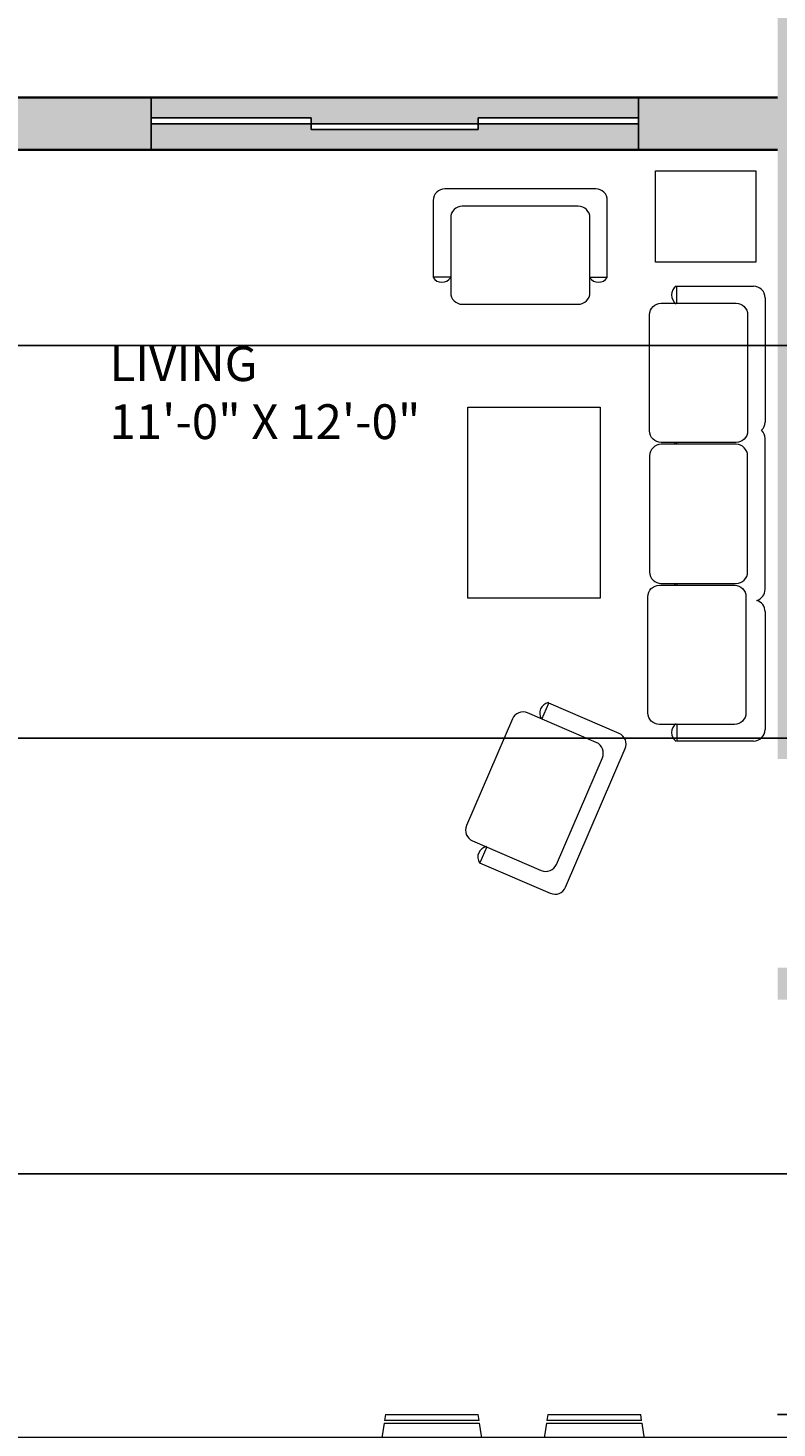
# Model space of a CAD drawing. Units: inches. Extents: x 1693 to 2974, y 2201 to 2965.
# Tile 21 of 24: x 2628 to 2757, y 2588 to 2829. Entities that reach past the tile are written whole.
import ezdxf

# ---------------------------------------------------------------- set-up
doc = ezdxf.new("R2010")
doc.units = ezdxf.units.IN
doc.header["$LTSCALE"] = 2
doc.header["$MEASUREMENT"] = 0
for name, color, linetype, lineweight in [('A-ANNO-DIMS', 2, 'Continuous', 18), ('A-AREA-IDEN', 7, 'Continuous', 18), ('A-DOOR', 3, 'Continuous', 25), ('A-FURN', 8, 'Continuous', 18), ('A-WALL', 7, 'Continuous', 35)]:
    doc.layers.add(name, color=color, linetype=linetype, lineweight=lineweight)
doc.layers.add('A-GLAZ-PATT', color=141, linetype='Continuous', lineweight=13, true_color=0xadddf7)
doc.layers.add('A-WALL-PATT', color=251, linetype='Continuous', lineweight=13, true_color=0x636466)
doc.styles.get("Standard").update_dxf_attribs({"font": 'arial.ttf'})
doc.dimstyles.get("Standard").update_dxf_attribs({"dimtxt": 0.18, "dimasz": 0.18, "dimexe": 0.18, "dimexo": 0.0625, "dimgap": 0.09, "dimtad": 0, "dimtih": 1, "dimtoh": 1, "dimdec": 1, "dimzin": 0, "dimdsep": 46, "dimlunit": 3, "dimtxsty": 'Standard', "dimcen": 0.09, "dimadec": 0, "dimazin": 0, "dimtfac": 1, "dimtdec": 1, "dimtofl": 0, "dimtmove": 0, "dimatfit": 3, "dimfxl": 1, "dimtolj": 1, "dimtzin": 0, "dimarcsym": 0})

# ---------------------------------------------------------------- blocks, each defined once
blk = doc.blocks.new('DINING-SET-72x36-6-SEAT')
for p, q in [((23.27, 53.5), (22.02, 45.5)), ((23.27, 53.5), (39.74, 53.5)), ((23.5, 55), (23.34, 54)), ((39.66, 54), (23.35, 54)), ((23.5, 55), (39.5, 55)), ((39.66, 54), (39.5, 55)), ((40.98, 45.5), (39.73, 53.5)), ((51.27, 53.5), (50.02, 45.5)), ((51.27, 53.5), (67.74, 53.5)), ((51.5, 55), (51.34, 54)), ((67.66, 54), (51.35, 54)), ((51.5, 55), (67.5, 55)), ((67.66, 54), (67.5, 55)), ((68.98, 45.5), (67.73, 53.5)), ((81.5, 45.5), (9.5, 45.5)), ((9.5, 45.5), (9.5, 9.5)), ((81.5, 9.5), (81.5, 45.5)), ((1.5, 35.73), (9.5, 36.98)), ((89.5, 35.73), (81.5, 36.98)), ((0, 35.5), (1, 35.66)), ((0, 35.5), (0, 19.5)), ((1, 19.34), (1, 35.65)), ((1.5, 35.73), (1.5, 19.26)), ((89.5, 35.73), (89.5, 19.26)), ((91, 35.5), (90, 35.66)), ((90, 19.34), (90, 35.65)), ((91, 35.5), (91, 19.5)), ((1, 19.34), (0, 19.5)), ((90, 19.34), (91, 19.5)), ((9.5, 18.02), (1.5, 19.27)), ((81.5, 18.02), (89.5, 19.27)), ((9.5, 9.5), (81.5, 9.5)), ((23.27, 1.5), (22.02, 9.5)), ((40.98, 9.5), (39.73, 1.5)), ((51.27, 1.5), (50.02, 9.5)), ((68.98, 9.5), (67.73, 1.5)), ((23.27, 1.5), (39.74, 1.5)), ((23.5, 0), (23.34, 1)), ((39.66, 1), (23.35, 1)), ((23.5, 0), (39.5, 0)), ((39.66, 1), (39.5, 0)), ((51.27, 1.5), (67.74, 1.5)), ((51.5, 0), (51.34, 1)), ((67.66, 1), (51.35, 1)), ((51.5, 0), (67.5, 0)), ((67.66, 1), (67.5, 0))]:
    blk.add_line(p, q)
blk = doc.blocks.new('*D62')
at = {"layer": 'A-ANNO-DIMS', "color": 0, "lineweight": -2, "ltscale": 2, "transparency": 16777216}
for p, q in [((2756.69, 2590.25), (2770.46, 2590.25)), ((2770.28, 2590.07), (2770.28, 2562.93)), ((2770.28, 2535.43), (2770.28, 2562.56)), ((2756.69, 2535.25), (2770.46, 2535.25))]:
    blk.add_line(p, q, dxfattribs=at)
at = {"layer": 'A-ANNO-DIMS', "color": 0, "ltscale": 2, "transparency": 16777216}
for points in [[(2770.25, 2590.07), (2770.31, 2590.07), (2770.28, 2590.25)], [(2770.25, 2535.43), (2770.31, 2535.43), (2770.28, 2535.25)]]:
    blk.add_solid(points, dxfattribs=at)
at = {"layer": 'Defpoints', "color": 0, "ltscale": 2, "transparency": 16777216}
for p in [(2756.63, 2590.25), (2770.28, 2590.25), (2756.63, 2535.25)]:
    blk.add_point(p, dxfattribs=at)
at = {"layer": 'A-ANNO-DIMS', "color": 0, "ltscale": 2, "transparency": 16777216, "insert": (2770.28, 2562.75), "char_height": 0.18, "attachment_point": 5}
blk.add_mtext('\\A1;55 TYP.', dxfattribs=at)
blk = doc.blocks.new('*D81')
at = {"layer": 'A-ANNO-DIMS', "color": 0, "lineweight": -2, "ltscale": 2, "transparency": 16777216}
for p, q in [((1752.34, 2553.91), (1752.34, 2964.96)), ((1752.52, 2964.78), (2332.94, 2964.78)), ((2914.06, 2964.78), (2333.64, 2964.78)), ((2914.24, 2754.97), (2914.24, 2964.96))]:
    blk.add_line(p, q, dxfattribs=at)
at = {"layer": 'A-ANNO-DIMS', "color": 0, "ltscale": 2, "transparency": 16777216}
for points in [[(1752.52, 2964.81), (1752.52, 2964.75), (1752.34, 2964.78)], [(2914.06, 2964.81), (2914.06, 2964.75), (2914.24, 2964.78)]]:
    blk.add_solid(points, dxfattribs=at)
at = {"layer": 'Defpoints', "color": 0, "ltscale": 2, "transparency": 16777216}
for p in [(2914.24, 2964.78), (2914.24, 2754.9), (1752.34, 2553.84)]:
    blk.add_point(p, dxfattribs=at)
at = {"layer": 'A-ANNO-DIMS', "color": 0, "ltscale": 2, "transparency": 16777216, "insert": (2333.29, 2964.78), "char_height": 0.18, "attachment_point": 5}
blk.add_mtext('\\A1;1162', dxfattribs=at)
blk = doc.blocks.new('*D90')
at = {"layer": 'A-ANNO-DIMS', "color": 0, "lineweight": -2, "ltscale": 2, "transparency": 16777216}
for p, q in [((2145.8, 2774.54), (2973.12, 2774.54)), ((2972.94, 2774.36), (2972.94, 2740.87)), ((2972.94, 2707.02), (2972.94, 2740.51)), ((2294.3, 2706.84), (2973.12, 2706.84))]:
    blk.add_line(p, q, dxfattribs=at)
at = {"layer": 'A-ANNO-DIMS', "color": 0, "ltscale": 2, "transparency": 16777216}
for points in [[(2972.91, 2774.36), (2972.97, 2774.36), (2972.94, 2774.54)], [(2972.91, 2707.02), (2972.97, 2707.02), (2972.94, 2706.84)]]:
    blk.add_solid(points, dxfattribs=at)
at = {"layer": 'Defpoints', "color": 0, "ltscale": 2, "transparency": 16777216}
for p in [(2145.74, 2774.54), (2294.24, 2706.84), (2972.94, 2706.84)]:
    blk.add_point(p, dxfattribs=at)
at = {"layer": 'A-ANNO-DIMS', "color": 0, "ltscale": 2, "transparency": 16777216, "insert": (2972.94, 2740.69), "char_height": 0.18, "attachment_point": 5}
blk.add_mtext('\\A1;67.7', dxfattribs=at)
blk = doc.blocks.new('*D97')
at = {"layer": 'A-ANNO-DIMS', "color": 0, "lineweight": -2, "ltscale": 2, "transparency": 16777216}
for p, q in [((2294.3, 2631.75), (2973.12, 2631.75)), ((2972.94, 2631.57), (2972.94, 2609.19)), ((2972.94, 2586.44), (2972.94, 2608.83)), ((2294.3, 2586.26), (2973.12, 2586.26))]:
    blk.add_line(p, q, dxfattribs=at)
at = {"layer": 'A-ANNO-DIMS', "color": 0, "ltscale": 2, "transparency": 16777216}
for points in [[(2972.91, 2631.57), (2972.97, 2631.57), (2972.94, 2631.75)], [(2972.91, 2586.44), (2972.97, 2586.44), (2972.94, 2586.26)]]:
    blk.add_solid(points, dxfattribs=at)
at = {"layer": 'Defpoints', "color": 0, "ltscale": 2, "transparency": 16777216}
for p in [(2294.24, 2631.75), (2972.94, 2631.75), (2294.24, 2586.26)]:
    blk.add_point(p, dxfattribs=at)
at = {"layer": 'A-ANNO-DIMS', "color": 0, "ltscale": 2, "transparency": 16777216, "insert": (2972.94, 2609.01), "char_height": 0.18, "attachment_point": 5}
blk.add_mtext('\\A1;45.49', dxfattribs=at)

msp = doc.modelspace()

# ---------------------------------------------------------------- hatches: boundary and pattern name
at = {"layer": 'A-GLAZ-PATT', "ltscale": 2}
h = msp.add_hatch(color=256, dxfattribs=at)
h.dxf.hatch_style = 1
h.paths.add_polyline_path([(2656.9702, 2338.2547), (2632.9702, 2338.2547), (2632.9702, 2339.2547), (2608.9702, 2339.2547), (2608.9702, 2334.7547), (2656.9702, 2334.7547)])
h.paths.add_polyline_path([(2656.9702, 2343.7547), (2608.9702, 2343.7547), (2608.9702, 2340.2547), (2632.9702, 2340.2547), (2632.9702, 2339.2547), (2656.9702, 2339.2547)])
h.paths.add_polyline_path([(2775.7544, 2338.2547), (2751.7544, 2338.2547), (2751.7544, 2334.7547), (2775.7544, 2334.7547)])
h.paths.add_polyline_path([(2775.7544, 2343.7547), (2751.7544, 2343.7547), (2751.7544, 2340.2547), (2775.7544, 2340.2547)])
h.paths.add_polyline_path([(2897.7363, 2568.7999), (2893.2363, 2568.7999), (2893.2363, 2520.7999), (2896.7363, 2520.7999), (2896.7363, 2544.7999), (2897.7363, 2544.7999)])
h.paths.add_polyline_path([(2902.2363, 2568.7999), (2898.7363, 2568.7999), (2898.7363, 2544.7999), (2897.7363, 2544.7999), (2897.7363, 2520.7999), (2902.2363, 2520.7999)])
h.paths.add_polyline_path([(2902.2363, 2637.7547), (2898.7363, 2637.7547), (2898.7363, 2613.7547), (2902.2363, 2613.7547)])
h.paths.add_polyline_path([(2896.7363, 2637.7547), (2893.2363, 2637.7547), (2893.2363, 2613.7547), (2896.7363, 2613.7547)])
h.paths.add_polyline_path([(2902.2363, 2748.903), (2899.0477, 2748.903), (2899.0477, 2724.903), (2898.0477, 2724.903), (2898.0477, 2700.903), (2902.2363, 2700.903)])
h.paths.add_polyline_path([(2898.0477, 2748.903), (2893.2363, 2748.903), (2893.2363, 2700.903), (2897.0477, 2700.903), (2897.0477, 2724.903), (2898.0477, 2724.903)])
h.paths.add_polyline_path([(2851.2363, 2846.2547), (2803.2363, 2846.2547), (2803.2363, 2842.7547), (2827.2363, 2842.7547), (2827.2363, 2841.7547), (2851.2363, 2841.7547)])
h.paths.add_polyline_path([(2851.2363, 2840.7547), (2827.2363, 2840.7547), (2827.2363, 2841.7547), (2803.2363, 2841.7547), (2803.2363, 2837.2547), (2851.2363, 2837.2547)])
h.paths.add_polyline_path([(2578.2363, 2846.2547), (2530.2363, 2846.2547), (2530.2363, 2842.7547), (2554.2363, 2842.7547), (2554.2363, 2841.7547), (2578.2363, 2841.7547)])
h.paths.add_polyline_path([(2578.2363, 2840.7547), (2554.2363, 2840.7547), (2554.2363, 2841.7547), (2530.2363, 2841.7547), (2530.2363, 2837.2547), (2578.2363, 2837.2547)])
h.paths.add_polyline_path([(2732.7363, 2812.7547), (2705.1363, 2812.7547), (2705.1363, 2811.7547), (2676.3363, 2811.7547), (2676.3363, 2812.7547), (2648.7363, 2812.7547), (2648.7363, 2808.2547), (2732.7363, 2808.2547)])
h.paths.add_polyline_path([(2732.7363, 2817.2547), (2648.7363, 2817.2547), (2648.7363, 2813.7547), (2676.3363, 2813.7547), (2676.3363, 2812.7547), (2705.1363, 2812.7547), (2705.1363, 2813.7547), (2732.7363, 2813.7547)])
h.paths.add_polyline_path([(2488.2363, 2695.8203), (2484.7878, 2695.8203), (2484.7878, 2671.8203), (2488.2363, 2671.8203)])
h.paths.add_polyline_path([(2482.7878, 2695.8203), (2479.2363, 2695.8203), (2479.2363, 2671.8203), (2482.7878, 2671.8203)])
h.paths.add_polyline_path([(2488.2363, 2572.4371), (2484.7363, 2572.4371), (2484.7363, 2541.4371), (2483.7363, 2541.4371), (2483.7363, 2512.4371), (2488.2363, 2512.4371)])
h.paths.add_polyline_path([(2482.7363, 2541.4371), (2483.7363, 2541.4371), (2483.7363, 2572.4371), (2479.2363, 2572.4371), (2479.2363, 2512.4371), (2482.7363, 2512.4371)])
h.paths.add_polyline_path([(2248.9863, 2706.8449), (2190.9863, 2706.8449), (2190.9863, 2703.3449), (2219.9863, 2703.3449), (2219.9863, 2702.3449), (2248.9863, 2702.3449)])
h.paths.add_polyline_path([(2248.9863, 2701.3449), (2219.9863, 2701.3449), (2219.9863, 2702.3449), (2190.9863, 2702.3449), (2190.9863, 2697.8449), (2248.9863, 2697.8449)])
h.paths.add_polyline_path([(2151.9207, 2293.3449), (2127.9207, 2293.3449), (2127.9207, 2289.8449), (2151.9207, 2289.8449)])
h.paths.add_polyline_path([(2151.9207, 2298.8449), (2127.9207, 2298.8449), (2127.9207, 2295.3449), (2151.9207, 2295.3449)])
h.paths.add_polyline_path([(2084.023, 2293.3449), (2066.023, 2293.3449), (2066.023, 2294.3449), (2048.023, 2294.3449), (2048.023, 2289.8449), (2084.023, 2289.8449)])
h.paths.add_polyline_path([(2084.023, 2298.8449), (2048.023, 2298.8449), (2048.023, 2295.3449), (2066.023, 2295.3449), (2066.023, 2294.3449), (2084.023, 2294.3449)])
h.paths.add_polyline_path([(1966.0781, 2293.3449), (1948.0781, 2293.3449), (1948.0781, 2294.3449), (1930.0781, 2294.3449), (1930.0781, 2289.8449), (1966.0781, 2289.8449)])
h.paths.add_polyline_path([(1966.0781, 2298.8449), (1930.0781, 2298.8449), (1930.0781, 2295.3449), (1948.0781, 2295.3449), (1948.0781, 2294.3449), (1966.0781, 2294.3449)])
h.paths.add_polyline_path([(1787.2363, 2403.1922), (1782.7363, 2403.1922), (1782.7363, 2355.1922), (1786.2363, 2355.1922), (1786.2363, 2379.1922), (1787.2363, 2379.1922)])
h.paths.add_polyline_path([(1791.7363, 2403.1922), (1788.2363, 2403.1922), (1788.2363, 2379.1922), (1787.2363, 2379.1922), (1787.2363, 2355.1922), (1791.7363, 2355.1922)])
h.paths.add_polyline_path([(1786.2363, 2477.5455), (1782.7363, 2477.5455), (1782.7363, 2453.5455), (1786.2363, 2453.5455)])
h.paths.add_polyline_path([(1791.7363, 2477.5455), (1788.2363, 2477.5455), (1788.2363, 2453.5455), (1791.7363, 2453.5455)])
h.paths.add_polyline_path([(1786.2363, 2621.6433), (1782.7363, 2621.6433), (1782.7363, 2585.6433), (1786.2363, 2585.6433)])
h.paths.add_polyline_path([(1791.7363, 2621.6433), (1788.2363, 2621.6433), (1788.2363, 2585.6433), (1791.7363, 2585.6433)])
h.paths.add_polyline_path([(1908.1286, 2706.8449), (1860.1286, 2706.8449), (1860.1286, 2703.3449), (1884.1286, 2703.3449), (1884.1286, 2702.3449), (1908.1286, 2702.3449)])
h.paths.add_polyline_path([(1908.1286, 2701.3449), (1884.1286, 2701.3449), (1884.1286, 2702.3449), (1860.1286, 2702.3449), (1860.1286, 2697.8449), (1908.1286, 2697.8449)])
h.paths.add_polyline_path([(1973.9863, 2706.8449), (1949.9863, 2706.8449), (1949.9863, 2703.3449), (1973.9863, 2703.3449)])
h.paths.add_polyline_path([(1973.9863, 2701.3449), (1949.9863, 2701.3449), (1949.9863, 2697.8449), (1973.9863, 2697.8449)])
h.paths.add_polyline_path([(2112.7363, 2690.3449), (2028.7363, 2690.3449), (2028.7363, 2686.8449), (2056.3363, 2686.8449), (2056.3363, 2685.8449), (2085.1363, 2685.8449), (2085.1363, 2686.8449), (2112.7363, 2686.8449)])
h.paths.add_polyline_path([(2112.7363, 2685.8449), (2085.1363, 2685.8449), (2085.1363, 2684.8449), (2056.3363, 2684.8449), (2056.3363, 2685.8449), (2028.7363, 2685.8449), (2028.7363, 2681.3449), (2112.7363, 2681.3449)])
h.paths.add_polyline_path([(2422.7363, 2640.7547), (2350.7363, 2640.7547), (2350.7363, 2637.2547), (2386.7363, 2637.2547), (2386.7363, 2636.2547), (2422.7363, 2636.2547)])
h.paths.add_polyline_path([(2422.7363, 2635.2547), (2386.7363, 2635.2547), (2386.7363, 2636.2547), (2350.7363, 2636.2547), (2350.7363, 2631.7547), (2422.7363, 2631.7547)])
at = {"layer": 'A-WALL-PATT', "ltscale": 2}
h = msp.add_hatch(color=256, dxfattribs=at)
h.dxf.hatch_style = 1
h.paths.add_polyline_path([(1928.2363, 2733.2161), (1930.9384, 2733.2161), (1930.9384, 2737.2161), (1923.7363, 2737.2161), (1923.7363, 2706.8449), (1908.1286, 2706.8449), (1908.1286, 2697.8449), (1923.7363, 2697.8449), (1923.7363, 2692.8449), (1928.2363, 2692.8449), (1928.2363, 2697.8449), (1949.9863, 2697.8449), (1949.9863, 2706.8449), (1928.2363, 2706.8449)])
h.paths.add_polyline_path([(2004.7363, 2737.2161), (1995.7363, 2737.2161), (1995.7363, 2706.8449), (1985.6374, 2706.8449), (1973.9863, 2706.8449), (1973.9863, 2697.8449), (2000.2363, 2697.8449), (2000.2363, 2686.5348), (2000.3613, 2686.5348), (2000.3613, 2667.0432), (2000.2363, 2601.8449), (1928.2363, 2601.8449), (1928.2363, 2662.8449), (1923.7363, 2662.8449), (1923.7363, 2595.3449), (1928.2363, 2595.3449), (1928.2363, 2597.3449), (2004.7363, 2597.3449), (2004.7363, 2681.3449), (2012.7814, 2681.3449), (2028.7363, 2681.3449), (2028.7363, 2690.3449), (2004.7363, 2690.3449)])
h.paths.add_polyline_path([(2190.9863, 2706.8449), (2184.9863, 2706.8449), (2145.7363, 2706.8449), (2145.7363, 2765.3449), (2145.7363, 2774.5394), (2136.7363, 2774.5394), (2136.7363, 2756.3449), (2136.7363, 2690.3449), (2112.7363, 2690.3449), (2112.7363, 2681.3449), (2136.7363, 2681.3449), (2136.7363, 2597.3449), (2141.2363, 2597.3449), (2141.2363, 2697.8449), (2190.9863, 2697.8449)])
h.paths.add_polyline_path([(1860.1286, 2706.8449), (1782.7363, 2706.8449), (1782.7363, 2621.6433), (1791.7363, 2621.6433), (1791.7363, 2697.8449), (1860.1286, 2697.8449)])
h.paths.add_polyline_path([(1791.7363, 2585.6433), (1782.7363, 2585.6433), (1782.7363, 2562.8449), (1782.7363, 2553.8449), (1752.3363, 2553.8449), (1752.3363, 2544.2586), (1756.3363, 2544.2586), (1756.3363, 2549.3449), (1782.7363, 2549.3449), (1782.7363, 2489.2404), (1782.7363, 2477.5455), (1791.7363, 2477.5455), (1791.7363, 2493.5991), (1791.6113, 2493.5991), (1791.6113, 2513.0907), (1791.6824, 2533.7198, -0.94742783), (1791.7363, 2534.7168), (1791.7363, 2549.3449), (1863.7363, 2549.3449), (1863.7363, 2513.3449), (1866.7363, 2513.3449), (1866.7363, 2549.3449), (1924.7363, 2549.3449), (1924.7363, 2447.3449), (1924.7363, 2442.8449), (1933.7363, 2442.8449), (1933.7363, 2447.3449), (1928.2363, 2447.3449), (1928.2363, 2559.3449), (1923.7363, 2559.3449), (1923.7363, 2553.8449), (1791.7363, 2553.8449), (1791.7363, 2562.8449)])
h.paths.add_polyline_path([(1791.7363, 2442.8449), (1866.7363, 2442.8449), (1866.7363, 2447.3449), (1866.7363, 2483.3449), (1863.7363, 2483.3449), (1863.7363, 2447.3449), (1791.7363, 2447.3449), (1791.7363, 2453.5455), (1782.7363, 2453.5455), (1782.7363, 2447.3449), (1756.3363, 2447.3449), (1756.3363, 2455.7126), (1752.3363, 2455.7126), (1752.3363, 2442.8449), (1782.7363, 2442.8449), (1782.7363, 2403.1922), (1791.7363, 2403.1922)])
h.paths.add_polyline_path([(1930.0781, 2298.8449), (1791.7363, 2298.8449), (1791.7363, 2355.1922), (1782.7363, 2355.1922), (1782.7363, 2289.8449), (1930.0781, 2289.8449)])
h.paths.add_polyline_path([(2624.7363, 2883.2547), (2624.7363, 2902.6165), (2624.7363, 2906.0761), (2615.7363, 2906.0761), (2615.7363, 2892.2547), (2615.7363, 2846.2547), (2578.2363, 2846.2547), (2578.2363, 2837.2547), (2620.2363, 2837.2547), (2620.2363, 2743.2547), (2624.7363, 2743.2547), (2624.7363, 2808.2547), (2648.7363, 2808.2547), (2648.7363, 2817.2547), (2624.7363, 2817.2547)])
h.paths.add_polyline_path([(2530.2363, 2846.2547), (2479.2363, 2846.2547), (2479.2363, 2695.8203), (2488.2363, 2695.8203), (2488.2363, 2700.7547), (2567.2363, 2700.7547), (2567.2363, 2705.2547), (2488.2363, 2705.2547), (2488.2363, 2837.2547), (2530.2363, 2837.2547)])
h.paths.add_polyline_path([(2488.2363, 2487.7547), (2630.2363, 2487.7547, -0.00990191), (2630.2363, 2489.0322), (2630.2363, 2492.2547), (2488.2363, 2492.2547), (2488.2363, 2512.4371), (2479.2363, 2512.4371), (2479.2363, 2334.7547), (2608.9702, 2334.7547), (2608.9702, 2343.7547), (2488.2363, 2343.7547)])
h.paths.add_polyline_path([(2751.7544, 2343.7547), (2672.7363, 2343.7547), (2672.7363, 2409.7547), (2674.7363, 2409.7547), (2674.7363, 2413.7547), (2672.7363, 2413.7547), (2672.7363, 2487.7547), (2732.7363, 2487.7547), (2732.7363, 2413.7547), (2704.7363, 2413.7547), (2704.7363, 2409.7547), (2784.7363, 2409.7547), (2784.7363, 2343.7547), (2775.7544, 2343.7547), (2775.7544, 2334.7547), (2902.2363, 2334.7547), (2902.2363, 2520.7999), (2893.2363, 2520.7999), (2893.2363, 2413.7547), (2856.0145, 2413.7547), (2856.0145, 2409.7547), (2893.2363, 2409.7547), (2893.2363, 2343.7547), (2789.2363, 2343.7547), (2789.2363, 2409.7547), (2819.2363, 2409.7547), (2826.0145, 2409.7547), (2826.0145, 2413.7547), (2789.2363, 2413.7547), (2789.2363, 2492.2547), (2784.7363, 2492.2547), (2784.7363, 2413.7547), (2736.7363, 2413.7547), (2736.7363, 2492.2547), (2672.7363, 2492.2547), (2666.2363, 2492.2547), (2666.2363, 2487.7547), (2668.2363, 2487.7547), (2668.2363, 2343.7547), (2656.9702, 2343.7547), (2656.9702, 2334.7547), (2662.9702, 2334.7547), (2751.7544, 2334.7547)])
h.paths.add_polyline_path([(2902.2363, 2613.7547), (2893.2363, 2613.7547), (2893.2363, 2589.7547), (2785.2363, 2589.7547), (2785.2363, 2661.7547), (2790.2363, 2661.7547), (2790.2363, 2665.2547), (2761.2363, 2665.2547), (2761.2363, 2667.2547), (2756.7363, 2667.2547), (2756.7363, 2661.7547), (2781.2363, 2661.7547), (2781.2363, 2585.7547), (2893.2363, 2585.7547), (2893.2363, 2568.7999), (2902.2363, 2568.7999)])
h.paths.add_polyline_path([(2488.2363, 2671.8203), (2479.2363, 2671.8203), (2479.2363, 2645.2547), (2479.2363, 2623.4598), (2488.2363, 2623.4598), (2488.2363, 2636.2547), (2624.7363, 2636.2547), (2624.7363, 2640.7547), (2603.7363, 2640.7547), (2603.7363, 2700.7547), (2624.7363, 2700.7547), (2624.7363, 2707.2547), (2620.2363, 2707.2547), (2620.2363, 2705.2547), (2597.2363, 2705.2547), (2597.2363, 2700.7547), (2599.2363, 2700.7547), (2599.2363, 2640.7547), (2488.2363, 2640.7547)])
h.paths.add_polyline_path([(2761.2363, 2837.2547), (2803.2363, 2837.2547), (2803.2363, 2846.2547), (2797.2363, 2846.2547), (2765.7363, 2846.2547), (2756.7363, 2846.2547), (2756.7363, 2817.2547), (2732.7363, 2817.2547), (2732.7363, 2808.2547), (2756.7363, 2808.2547), (2756.7363, 2703.2547), (2761.2363, 2703.2547)])
h.paths.add_polyline_path([(2739.7489, 2433.1234), (2786.9181, 2433.1234), (2786.9181, 2455.5122), (2739.7489, 2455.5122)], flags=25)

# ---------------------------------------------------------------- linework, layer by layer
at = {"layer": 'A-DOOR', "ltscale": 2}
for p, q in [((2648.7363, 2817.2547), (2648.7363, 2808.2547)), ((2732.7363, 2817.2547), (2732.7363, 2808.2547)), ((2648.7363, 2813.7547), (2676.3363, 2813.7547)), ((2648.7363, 2812.7547), (2732.7363, 2812.7547)), ((2676.3363, 2813.7547), (2676.3363, 2811.7547)), ((2676.3363, 2811.7547), (2705.1363, 2811.7547)), ((2705.1363, 2813.7547), (2705.1363, 2811.7547)), ((2705.1363, 2813.7547), (2732.7363, 2813.7547))]:
    msp.add_line(p, q, dxfattribs=at)
at = {"layer": 'A-FURN', "ltscale": 2}
for p, q in [((2700.373, 2786.3206), (2697.373, 2786.3206)), ((2724.3781, 2786.3206), (2727.3781, 2786.3206)), ((2739.2568, 2784.761), (2752.5638, 2784.761)), ((2739.3529, 2781.761), (2739.3529, 2784.761)), ((2754.5638, 2782.761), (2754.5638, 2761.3265)), ((2739.3529, 2757.4981), (2739.3529, 2757.8044)), ((2739.3529, 2733.4931), (2739.3529, 2733.2073)), ((2754.5638, 2728.6612), (2754.5638, 2708.3314)), ((2716.0967, 2710.1259), (2717.2831, 2712.8813)), ((2739.3529, 2709.3314), (2739.3529, 2706.3314)), ((2752.5638, 2706.3314), (2739.3529, 2706.3314)), ((2706.6038, 2688.0776), (2705.4175, 2685.3221))]:
    msp.add_line(p, q, dxfattribs=at)
for points in [[(2735.6536, 2804.6502), (2752.9928, 2804.6502), (2752.9928, 2788.9002), (2735.6536, 2788.9002)], [(2703.3147, 2763.8888), (2726.1354, 2763.8888), (2726.1354, 2730.9746), (2703.3147, 2730.9746)]]:
    msp.add_lwpolyline(points, close=True, dxfattribs=at)
for points in [[(2727.3781, 2786.2245), (2727.3781, 2799.5314, 0.41421356), (2725.3781, 2801.5314), (2699.373, 2801.5314, 0.41421356), (2697.373, 2799.5314), (2697.373, 2786.3206)], [(2722.3781, 2781.6361, 0.41421356), (2724.3781, 2783.6361), (2724.3781, 2796.5314, 0.41421356), (2722.3781, 2798.5314), (2702.373, 2798.5314, 0.41421356), (2700.373, 2796.5314), (2700.373, 2783.6361, 0.41421356), (2702.373, 2781.6361), (2722.3781, 2781.6361)], [(2734.6684, 2779.8094, -0.41421356), (2736.6684, 2781.8094), (2749.5638, 2781.8094, -0.41421356), (2751.5638, 2779.8094), (2751.5638, 2759.8044, -0.41421356), (2749.5638, 2757.8044), (2736.6684, 2757.8044, -0.41421356), (2734.6684, 2759.8044), (2734.6684, 2779.8094)], [(2753.1375, 2730.5771, 0.33134351), (2754.5638, 2732.4931), (2754.5638, 2758.4981, 0.19891237), (2753.978, 2759.9123)], [(2734.6684, 2735.4931, 0.41421356), (2736.6684, 2733.4931), (2749.5638, 2733.4931, 0.41421356), (2751.5638, 2735.4931), (2751.5638, 2755.4981, 0.41421356), (2749.5638, 2757.4981), (2736.6684, 2757.4981, 0.41421356), (2734.6684, 2755.4981), (2734.6684, 2735.4931)], [(2734.3774, 2731.2073, -0.41421356), (2736.3774, 2733.2073), (2749.2727, 2733.2073, -0.41421356), (2751.2727, 2731.2073), (2751.2727, 2711.2023, -0.41421356), (2749.2727, 2709.2023), (2736.3774, 2709.2023, -0.41421356), (2734.3774, 2711.2023), (2734.3774, 2731.2073)], [(2705.3292, 2685.3601), (2717.5514, 2680.0979, 0.41421356), (2720.1793, 2681.1439), (2730.4631, 2705.0292, 0.41421356), (2729.417, 2707.6571), (2717.2831, 2712.8813)], [(2703.0921, 2691.7671, 0.41421356), (2704.1381, 2689.1392), (2715.9823, 2684.0397, 0.41421356), (2718.6102, 2685.0858), (2726.5213, 2703.4601, 0.41421356), (2725.4752, 2706.088), (2713.631, 2711.1875, 0.41421356), (2711.0031, 2710.1414), (2703.0921, 2691.7671)]]:
    msp.add_lwpolyline(points, format="xyb", dxfattribs=at)
for centre, radius, start, end in [((2698.8506, 2787.2909), 1.8587, 215.008433, 324.991567), ((2725.8556, 2787.2909), 1.8587, 215.008433, 324.991567), ((2740.3232, 2783.2385), 1.8587, 125.008433, 234.991567), ((2752.5638, 2782.761), 2, 0, 90), ((2752.5638, 2761.3265), 2, 315, 0), ((2740.3232, 2759.0205), 1.8587, 220.865654, 234.991567), ((2740.3232, 2732.0155), 1.8587, 125.008433, 140.119023), ((2752.5638, 2728.6612), 2, 0, 73.32912), ((2717.5899, 2711.1405), 1.8587, 101.714199, 211.697334), ((2740.3232, 2707.809), 1.8587, 125.008433, 234.991567), ((2752.5638, 2708.3314), 2, 270, 0), ((2706.9107, 2686.3368), 1.8587, 101.714199, 211.697334)]:
    msp.add_arc(centre, radius, start, end, dxfattribs=at)
at = {"layer": 'A-WALL', "ltscale": 2}
for p, q in [((2624.7363, 2817.2547), (2756.7363, 2817.2547)), ((2624.7363, 2808.2547), (2756.7363, 2808.2547))]:
    msp.add_line(p, q, dxfattribs=at)

# ---------------------------------------------------------------- block references
at = {"layer": 'A-FURN'}
msp.add_blockref('DINING-SET-72x36-6-SEAT', (2665.6267, 2535.2453), dxfattribs=at)

# ---------------------------------------------------------------- texts
at = {"layer": 'A-AREA-IDEN', "ltscale": 2, "insert": (2641.5473, 2774.3918), "char_height": 6, "attachment_point": 1}
msp.add_mtext_dynamic_manual_height_columns('LIVING\\P11\'-0" X 12\'-0"', width=108.452746, gutter_width=1, heights=[0], dxfattribs=at)

# ---------------------------------------------------------------- dimensions: what is measured, and where the dimension line sits
at = {"layer": 'A-ANNO-DIMS', "ltscale": 2}
dim = msp.add_linear_dim(base=(2914.2363, 2964.7761), p1=(1752.3363, 2553.8449), p2=(2914.2363, 2754.903), dimstyle='Standard', override={"dimdec": 0, "dimlfac": 1, "dimrnd": 0, "dimzin": 0, "dimdsep": 46, "dimlunit": 2}, dxfattribs=at)
dim.commit()
dim.dimension.update_dxf_attribs({"geometry": '*D81', "text_midpoint": (2333.2863, 2964.7761)})
for base, p1, p2, override, picture, middle in [((2972.9363, 2706.8449), (2145.7363, 2774.5394), (2294.2363, 2706.8449), {"dimdec": 1, "dimlfac": 1, "dimrnd": 0, "dimzin": 0, "dimdsep": 46, "dimlunit": 2}, '*D90', (2972.9363, 2740.6922)), ((2972.9363, 2631.7547), (2294.2363, 2586.2648), (2294.2363, 2631.7547), {"dimdec": 2, "dimlfac": 1, "dimrnd": 0, "dimzin": 0, "dimdsep": 46, "dimlunit": 2}, '*D97', (2972.9363, 2609.0097))]:
    dim = msp.add_linear_dim(base=base, p1=p1, p2=p2, angle=90, dimstyle='Standard', override=override, dxfattribs=at)
    dim.commit()
    dim.dimension.update_dxf_attribs({"geometry": picture, "text_midpoint": middle})
dim = msp.add_linear_dim(base=(2770.2768, 2590.2455), p1=(2756.6268, 2535.2455), p2=(2756.6268, 2590.2455), angle=90, text='<> TYP.', dimstyle='Standard', override={"dimdec": 0, "dimlfac": 1, "dimrnd": 0, "dimzin": 0, "dimdsep": 46, "dimlunit": 2}, dxfattribs=at)
dim.commit()
dim.dimension.update_dxf_attribs({"geometry": '*D62', "text_midpoint": (2770.2768, 2562.7455)})

doc.saveas('drawing.dxf')
